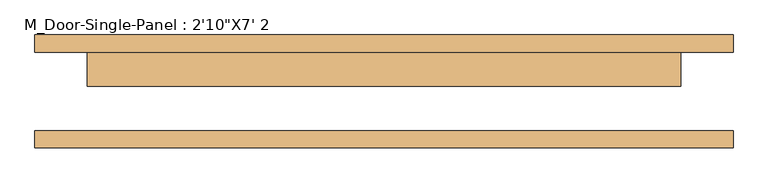
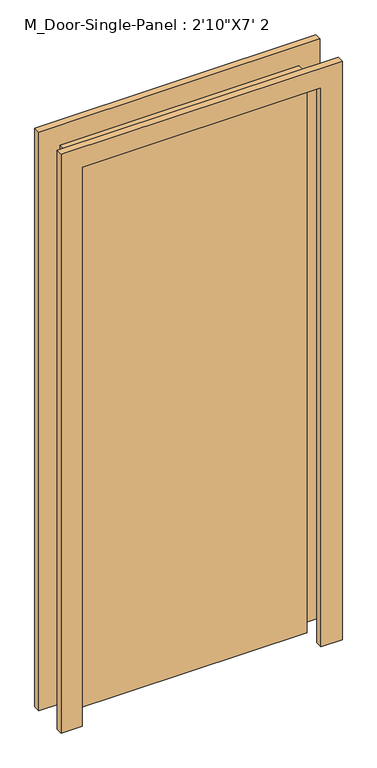
"""IFC4 building model written with IfcOpenShell, lengths in millimetres: door geometry."""

from ifc_helpers import new_model, si_unit, frame, origin, origin_with_axes, place, context, project, spatial, polyline, outline, extrude, source, transform, mapped, element, save


def door_07b5d71c(model_context):
    return source(origin(), model_context, "Body", "SweptSolid", [
        extrude(outline(polyline([(431.8, 7.15), (-431.8, 7.15), (-431.8, 57.15), (431.8, 57.15), (431.8, 7.15)])), origin_with_axes(), (0.0, 0.0, 1.0), 2133.6),
        extrude(outline(polyline([(2209.8, 508.0), (2209.8, -508.0), (0.0, -508.0), (0.0, -431.8), (2133.6, -431.8), (2133.6, 431.8), (0.0, 431.8), (0.0, 508.0), (2209.8, 508.0)])), frame((0.0, -82.15, 0.0), z_axis=(0.0, 1.0, 0.0), x_axis=(0.0, 0.0, 1.0)), (0.0, 0.0, 1.0), 25.0),
        extrude(outline(polyline([(2209.8, -508.0), (0.0, -508.0), (0.0, -431.8), (2133.6, -431.8), (2133.6, 431.8), (0.0, 431.8), (0.0, 508.0), (2209.8, 508.0), (2209.8, -508.0)])), frame((0.0, 57.15, 0.0), z_axis=(0.0, 1.0, 0.0), x_axis=(0.0, 0.0, 1.0)), (0.0, 0.0, 1.0), 25.0),
    ])


if __name__ == "__main__":
    model = new_model("IFC4")
    model_context = context("Model", 3, world=origin())
    ifc_project = project(units=[si_unit("LENGTHUNIT", "METRE", prefix="MILLI")], contexts=[model_context])
    site = spatial("IfcSite", under=ifc_project)
    building = spatial("IfcBuilding", under=site)
    placement = place(None, origin())
    door_shape = door_07b5d71c(model_context)
    element("IfcDoor", 1, ObjectType="M_Door-Single-Panel : 2'10\"X7' 2", at=placement, inside=building, context=model_context, shape_type="MappedRepresentation", body=[
        mapped(door_shape, transform((0.0, 0.0, 0.0), x_axis=(1.0, 0.0, 0.0), y_axis=(0.0, 1.0, 0.0), z_axis=(0.0, 0.0, 1.0))),
    ])
    save(model, "model.ifc")

# Revit data of these elements
# Type "M_Door-Single-Panel : 2'10\"X7' 2"
#   Type Mark = "10"
#   Construction Type Id = "DOOR"
#   Assembly Code = "C1020300"
#   Analytic Construction = "Wooden"
#   Thickness = 0' - 1.9685"
#   Thermal Resistance (R) = 2.5876 (h·ft²·°F)/BTU
#   Swing Angle [instance default] = 90.00°
#   Heat Transfer Coefficient (U) = 0.3865 BTU/(h·ft²·°F)
#   Height = 7' - 0"
#   Trim Projection Ext = 0' - 0.98425"
#   Trim Projection Int = 0' - 0.98425"
#   Trim Width = 0' - 3.14961"
#   Width = 2' - 10"
#   Define Thermal Properties by = 1
#   Panel Material = Wood - Birch - Solid Stained Light Low Gloss
#   Trim Material = Paint - Sienna
#   Visual Light Transmittance = 0
#   Solar Heat Gain Coefficient = 0
#   Function = (empty or 0)
#   Wall Closure = (empty or 0)
# Element 1 (IfcDoor, "M_Door-Single-Panel : 2'10\"X7' 2")
#   Materials on its faces: "Paint - Sienna", "Wood - Birch - Solid Stained Light Low Gloss"
# Materials
#   "Wood - Birch - Solid Stained Light Low Gloss": class "Wood", colour RGB 210 159 95, transparency 0, Cost = 0
#   "Paint - Sienna": colour RGB 118 70 51, transparency 0, Cost = 0
